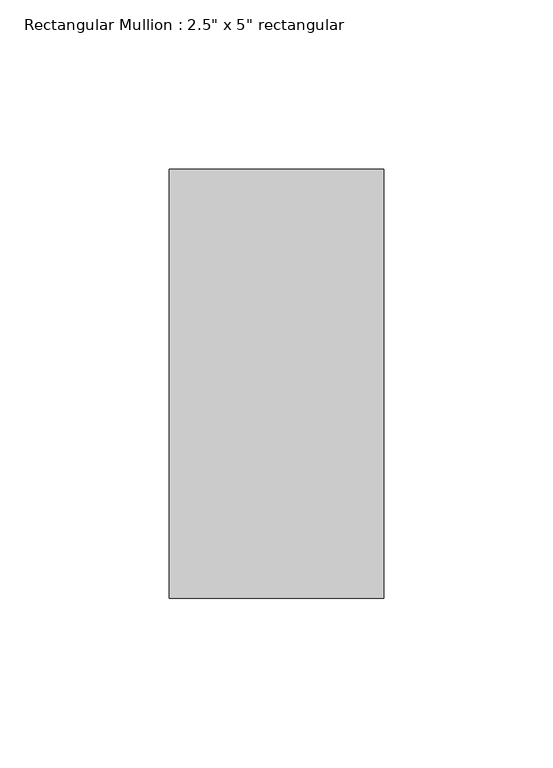
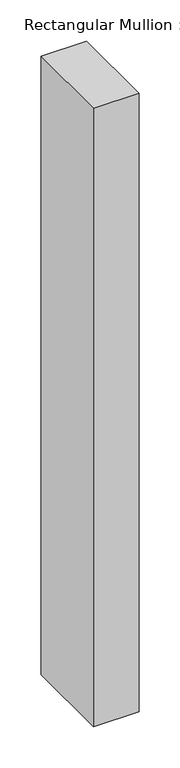
"""IFC4 building model written with IfcOpenShell, lengths in millimetres: member geometry."""

from ifc_helpers import new_model, si_unit, frame, origin, place, context, project, spatial, polyline, outline, extrude, source, transform, mapped, element, save


def member_62b9d9f2(model_context):
    return source(origin(), model_context, "Body", "SweptSolid", [
        extrude(outline(polyline([(31.75, 63.5), (31.75, -63.5), (-31.75, -63.5), (-31.75, 63.5), (31.75, 63.5)])), frame((0.0, 0.0, -914.0980012), z_axis=(0.0, 0.0, 1.0), x_axis=(1.0, 0.0, 0.0)), (0.0, 0.0, 1.0), 914.0980012),
    ])


if __name__ == "__main__":
    model = new_model("IFC4")
    model_context = context("Model", 3, world=origin())
    ifc_project = project(units=[si_unit("LENGTHUNIT", "METRE", prefix="MILLI")], contexts=[model_context])
    site = spatial("IfcSite", under=ifc_project)
    building = spatial("IfcBuilding", under=site)
    placement = place(None, origin())
    member_shape = member_62b9d9f2(model_context)
    element("IfcMember", 1, ObjectType="Rectangular Mullion : 2.5\" x 5\" rectangular", at=placement, inside=building, context=model_context, shape_type="MappedRepresentation", body=[
        mapped(member_shape, transform((0.0, 0.0, 0.0), x_axis=(1.0, 0.0, 0.0), y_axis=(0.0, 1.0, 0.0), z_axis=(0.0, 0.0, 1.0))),
    ])
    save(model, "model.ifc")

# Revit data of these elements
# Type "Rectangular Mullion : 2.5\" x 5\" rectangular"
#   built-in parameter 1007304 = 0.416667 (stored number, unit not read)
#   built-in parameter 1007301 = 0.104167 (stored number, unit not read)
#   built-in parameter 1007300 = 0.104167 (stored number, unit not read)
# Element 1 (IfcMember, "Rectangular Mullion : 2.5\" x 5\" rectangular")
#   Materials on its faces: "Aluminum"
# Materials
#   "Aluminum": class "Metal", colour RGB 247 247 247, transparency 0, Description = "Aluminum 6061", Cost = 0
